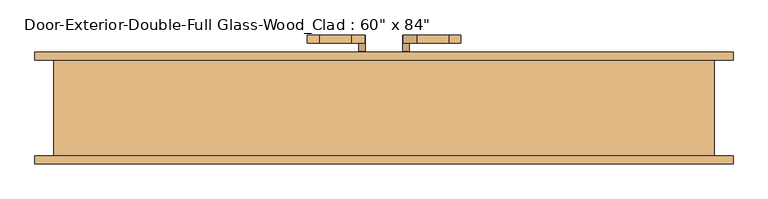
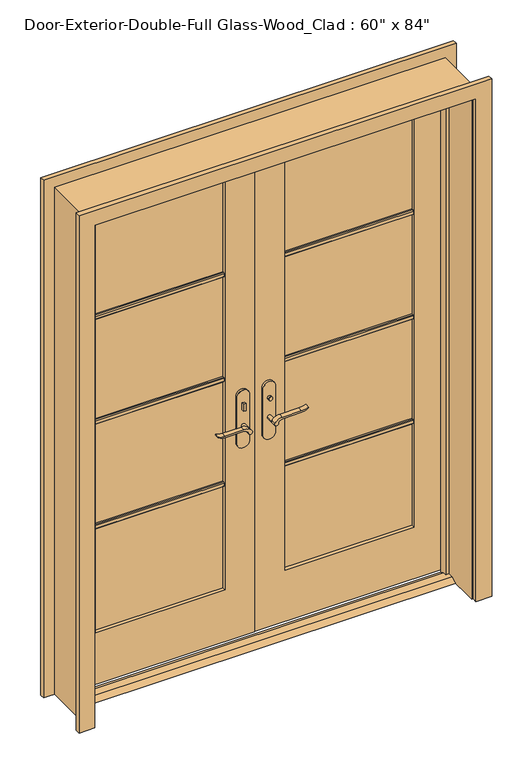
"""IFC4 building model written with IfcOpenShell, lengths in millimetres: door geometry."""

from ifc_helpers import new_model, si_unit, point, frame, frame_2d, origin, place, context, project, spatial, polyline, circle_curve, trimmed, segment, composite_curve, outline, extrude, faceted_brep, source, transform, mapped, element, save


def door_7ffae4ec(model_context):
    return source(origin(), model_context, "Body", "SolidModel", [
        extrude(outline(polyline([(19.05, 12.7), (53.975, 12.7), (79.375, 0.0), (-6.35, 0.0), (19.05, 12.7)])), frame((-762.0, 0.0, 0.0), z_axis=(1.0, 0.0, 0.0), x_axis=(0.0, 1.0, 0.0)), (0.0, 0.0, 1.0), 1524.0),
        extrude(outline(polyline([(-47.4019111, 56.2), (-57.4019111, 56.2), (-57.4019111, 66.2), (-47.4019111, 66.2), (-47.4019111, 56.2)])), frame((0.0, 0.0, 981.9), z_axis=(0.0, 0.0, 1.0), x_axis=(1.0, 0.0, 0.0)), (0.0, 0.0, 1.0), 30.0),
        extrude(outline(composite_curve([segment(trimmed(circle_curve(frame_2d((996.9, -52.4019111)), 8.0), [point((996.9, -60.4019111))], [point((996.9, -44.4019111))], False, "CARTESIAN"), True, "CONTINUOUS"), segment(trimmed(circle_curve(frame_2d((996.9, -52.4019111)), 8.0), [point((996.9, -44.4019111))], [point((996.9, -60.4019111))], False, "CARTESIAN"), True, "CONTINUOUS")], self_intersect=False)), frame((0.0, 121.125, 0.0), z_axis=(0.0, 1.0, 0.0), x_axis=(0.0, 0.0, 1.0)), (0.0, 0.0, 1.0), 10.0),
        extrude(outline(composite_curve([segment(trimmed(circle_curve(frame_2d((897.1555521, -76.0694241)), 37.2832219), [point((919.0523287, -45.8937749))], [point((934.4, -77.7693445))], False, "CARTESIAN"), True, "CONTINUOUS"), segment(polyline([(934.4, -77.7693445), (934.4, -154.045502)]), True, "CONTINUOUS"), segment(trimmed(circle_curve(frame_2d((1017.6850638, -153.9791202)), 83.2850902), [point((934.4, -154.045502))], [point((939.4, -182.4019111))], True, "CARTESIAN"), True, "CONTINUOUS"), segment(polyline([(939.4, -182.4019111), (936.6135558, -182.4019111)]), True, "CONTINUOUS"), segment(trimmed(circle_curve(frame_2d((986.6709207, -150.4622499)), 59.3791355), [point((936.6135558, -182.4019111))], [point((927.4, -154.045502))], False, "CARTESIAN"), True, "CONTINUOUS"), segment(polyline([(927.4, -154.045502), (927.4, -77.7881013)]), True, "CONTINUOUS"), segment(trimmed(circle_curve(frame_2d((909.2738613, -77.7881013)), 18.1261387), [point((927.4, -77.7881013))], [point((914.4, -60.4019111))], True, "CARTESIAN"), True, "CONTINUOUS"), segment(trimmed(circle_curve(frame_2d((914.4, -52.4019111)), 8.0), [point((914.4, -60.4019111))], [point((919.0523287, -45.8937749))], False, "CARTESIAN"), True, "CONTINUOUS")], self_intersect=False)), frame((0.0, 16.2, 0.0), z_axis=(0.0, 1.0, 0.0), x_axis=(0.0, 0.0, 1.0)), (0.0, 0.0, 1.0), 20.0),
        extrude(outline(composite_curve([segment(trimmed(circle_curve(frame_2d((914.4, -52.4019111)), 8.0), [point((914.3999903, -60.4019111))], [point((919.0523287, -45.8937749))], False, "CARTESIAN"), True, "CONTINUOUS"), segment(trimmed(circle_curve(frame_2d((897.1555521, -76.0694241)), 37.2832219), [point((919.0523287, -45.8937749))], [point((934.4, -77.7693445))], False, "CARTESIAN"), True, "CONTINUOUS"), segment(polyline([(934.4, -77.7693445), (934.4, -154.045502)]), True, "CONTINUOUS"), segment(trimmed(circle_curve(frame_2d((1017.6850638, -153.9791202)), 83.2850902), [point((934.4, -154.045502))], [point((939.4, -182.4019111))], True, "CARTESIAN"), True, "CONTINUOUS"), segment(polyline([(939.4, -182.4019111), (936.6135558, -182.4019111)]), True, "CONTINUOUS"), segment(trimmed(circle_curve(frame_2d((986.6709207, -150.4622499)), 59.3791355), [point((936.6135558, -182.4019111))], [point((927.4, -154.045502))], False, "CARTESIAN"), True, "CONTINUOUS"), segment(polyline([(927.4, -154.045502), (927.4, -77.788099)]), True, "CONTINUOUS"), segment(trimmed(circle_curve(frame_2d((909.2738682, -77.788099)), 18.1261318), [point((927.4, -77.788099))], [point((914.3999903, -60.4019111))], True, "CARTESIAN"), True, "CONTINUOUS")], self_intersect=False)), frame((0.0, 151.125, 0.0), z_axis=(0.0, 1.0, 0.0), x_axis=(0.0, 0.0, 1.0)), (0.0, 0.0, 1.0), 20.0),
        extrude(outline(composite_curve([segment(trimmed(circle_curve(frame_2d((914.4, -52.4019111)), 8.0), [point((914.4, -60.4019111))], [point((914.4, -44.4019111))], False, "CARTESIAN"), True, "CONTINUOUS"), segment(trimmed(circle_curve(frame_2d((914.4, -52.4019111)), 8.0), [point((914.4, -44.4019111))], [point((914.4, -60.4019111))], False, "CARTESIAN"), True, "CONTINUOUS")], self_intersect=False)), frame((0.0, 36.2, 0.0), z_axis=(0.0, 1.0, 0.0), x_axis=(0.0, 0.0, 1.0)), (0.0, 0.0, 1.0), 30.0),
        extrude(outline(composite_curve([segment(trimmed(circle_curve(frame_2d((914.4, -52.4019111)), 8.0), [point((914.4, -60.4019111))], [point((914.4, -44.4019111))], False, "CARTESIAN"), True, "CONTINUOUS"), segment(trimmed(circle_curve(frame_2d((914.4, -52.4019111)), 8.0), [point((914.4, -44.4019111))], [point((914.4, -60.4019111))], False, "CARTESIAN"), True, "CONTINUOUS")], self_intersect=False)), frame((0.0, 121.125, 0.0), z_axis=(0.0, 1.0, 0.0), x_axis=(0.0, 0.0, 1.0)), (0.0, 0.0, 1.0), 30.0),
        extrude(outline(composite_curve([segment(polyline([(844.4, -27.4019111), (1039.4, -27.4019111)]), True, "CONTINUOUS"), segment(trimmed(circle_curve(frame_2d((1039.4, -52.4019111)), 25.0), [point((1039.4, -27.4019111))], [point((1039.4, -77.4019111))], False, "CARTESIAN"), True, "CONTINUOUS"), segment(polyline([(1039.4, -77.4019111), (844.4, -77.4019111)]), True, "CONTINUOUS"), segment(trimmed(circle_curve(frame_2d((844.4, -52.4019111)), 25.0), [point((844.4, -77.4019111))], [point((844.4, -27.4019111))], False, "CARTESIAN"), True, "CONTINUOUS")], self_intersect=False)), frame((0.0, 66.2, 0.0), z_axis=(0.0, 1.0, 0.0), x_axis=(0.0, 0.0, 1.0)), (0.0, 0.0, 1.0), 10.0),
        extrude(outline(composite_curve([segment(polyline([(844.4, -27.4019111), (1039.4, -27.4019111)]), True, "CONTINUOUS"), segment(trimmed(circle_curve(frame_2d((1039.4, -52.4019111)), 25.0), [point((1039.4, -27.4019111))], [point((1039.4, -77.4019111))], False, "CARTESIAN"), True, "CONTINUOUS"), segment(polyline([(1039.4, -77.4019111), (844.4, -77.4019111)]), True, "CONTINUOUS"), segment(trimmed(circle_curve(frame_2d((844.4, -52.4019111)), 25.0), [point((844.4, -77.4019111))], [point((844.4, -27.4019111))], False, "CARTESIAN"), True, "CONTINUOUS")], self_intersect=False)), frame((0.0, 111.125, 0.0), z_axis=(0.0, 1.0, 0.0), x_axis=(0.0, 0.0, 1.0)), (0.0, 0.0, 1.0), 10.0),
        extrude(outline(polyline([(47.3875, 131.125), (57.3875, 131.125), (57.3875, 121.125), (47.3875, 121.125), (47.3875, 131.125)])), frame((0.0, 0.0, 981.9), z_axis=(0.0, 0.0, 1.0), x_axis=(1.0, 0.0, 0.0)), (0.0, 0.0, 1.0), 30.0),
        extrude(outline(composite_curve([segment(trimmed(circle_curve(frame_2d((996.9, 52.3875)), 8.0), [point((996.9, 60.3875))], [point((996.9, 44.3875))], False, "CARTESIAN"), True, "CONTINUOUS"), segment(trimmed(circle_curve(frame_2d((996.9, 52.3875)), 8.0), [point((996.9, 44.3875))], [point((996.9, 60.3875))], False, "CARTESIAN"), True, "CONTINUOUS")], self_intersect=False)), frame((0.0, 56.2, 0.0), z_axis=(0.0, 1.0, 0.0), x_axis=(0.0, 0.0, 1.0)), (0.0, 0.0, 1.0), 10.0),
        extrude(outline(composite_curve([segment(trimmed(circle_curve(frame_2d((914.4, 52.3875)), 8.0), [point((919.0523287, 45.8793637))], [point((914.4, 60.3875))], False, "CARTESIAN"), True, "CONTINUOUS"), segment(trimmed(circle_curve(frame_2d((909.2738613, 77.7736901)), 18.1261387), [point((914.4, 60.3875))], [point((927.4, 77.7736901))], True, "CARTESIAN"), True, "CONTINUOUS"), segment(polyline([(927.4, 77.7736901), (927.4, 154.0310909)]), True, "CONTINUOUS"), segment(trimmed(circle_curve(frame_2d((986.6709207, 150.4478388)), 59.3791355), [point((927.4, 154.0310909))], [point((936.6135558, 182.3875))], False, "CARTESIAN"), True, "CONTINUOUS"), segment(polyline([(936.6135558, 182.3875), (939.4, 182.3875)]), True, "CONTINUOUS"), segment(trimmed(circle_curve(frame_2d((1017.6850638, 153.9647091)), 83.2850902), [point((939.4, 182.3875))], [point((934.4, 154.0310909))], True, "CARTESIAN"), True, "CONTINUOUS"), segment(polyline([(934.4, 154.0310909), (934.4, 77.7549333)]), True, "CONTINUOUS"), segment(trimmed(circle_curve(frame_2d((897.1555521, 76.0550129)), 37.2832219), [point((934.4, 77.7549333))], [point((919.0523287, 45.8793637))], False, "CARTESIAN"), True, "CONTINUOUS")], self_intersect=False)), frame((0.0, 151.125, 0.0), z_axis=(0.0, 1.0, 0.0), x_axis=(0.0, 0.0, 1.0)), (0.0, 0.0, 1.0), 20.0),
        extrude(outline(composite_curve([segment(trimmed(circle_curve(frame_2d((909.2738682, 77.7736878)), 18.1261318), [point((914.3999903, 60.3875))], [point((927.4, 77.7736878))], True, "CARTESIAN"), True, "CONTINUOUS"), segment(polyline([(927.4, 77.7736878), (927.4, 154.0310909)]), True, "CONTINUOUS"), segment(trimmed(circle_curve(frame_2d((986.6709207, 150.4478388)), 59.3791355), [point((927.4, 154.0310909))], [point((936.6135558, 182.3875))], False, "CARTESIAN"), True, "CONTINUOUS"), segment(polyline([(936.6135558, 182.3875), (939.4, 182.3875)]), True, "CONTINUOUS"), segment(trimmed(circle_curve(frame_2d((1017.6850638, 153.9647091)), 83.2850902), [point((939.4, 182.3875))], [point((934.4, 154.0310909))], True, "CARTESIAN"), True, "CONTINUOUS"), segment(polyline([(934.4, 154.0310909), (934.4, 77.7549333)]), True, "CONTINUOUS"), segment(trimmed(circle_curve(frame_2d((897.1555521, 76.0550129)), 37.2832219), [point((934.4, 77.7549333))], [point((919.0523287, 45.8793637))], False, "CARTESIAN"), True, "CONTINUOUS"), segment(trimmed(circle_curve(frame_2d((914.4, 52.3875)), 8.0), [point((919.0523287, 45.8793637))], [point((914.3999903, 60.3875))], False, "CARTESIAN"), True, "CONTINUOUS")], self_intersect=False)), frame((0.0, 16.2, 0.0), z_axis=(0.0, 1.0, 0.0), x_axis=(0.0, 0.0, 1.0)), (0.0, 0.0, 1.0), 20.0),
        extrude(outline(composite_curve([segment(trimmed(circle_curve(frame_2d((914.4, 52.3875)), 8.0), [point((914.4, 60.3875))], [point((914.4, 44.3875))], False, "CARTESIAN"), True, "CONTINUOUS"), segment(trimmed(circle_curve(frame_2d((914.4, 52.3875)), 8.0), [point((914.4, 44.3875))], [point((914.4, 60.3875))], False, "CARTESIAN"), True, "CONTINUOUS")], self_intersect=False)), frame((0.0, 121.125, 0.0), z_axis=(0.0, 1.0, 0.0), x_axis=(0.0, 0.0, 1.0)), (0.0, 0.0, 1.0), 30.0),
        extrude(outline(composite_curve([segment(trimmed(circle_curve(frame_2d((914.4, 52.3875)), 8.0), [point((914.4, 60.3875))], [point((914.4, 44.3875))], False, "CARTESIAN"), True, "CONTINUOUS"), segment(trimmed(circle_curve(frame_2d((914.4, 52.3875)), 8.0), [point((914.4, 44.3875))], [point((914.4, 60.3875))], False, "CARTESIAN"), True, "CONTINUOUS")], self_intersect=False)), frame((0.0, 36.2, 0.0), z_axis=(0.0, 1.0, 0.0), x_axis=(0.0, 0.0, 1.0)), (0.0, 0.0, 1.0), 30.0),
        extrude(outline(composite_curve([segment(trimmed(circle_curve(frame_2d((844.4, 52.3875)), 25.0), [point((844.4, 27.3875))], [point((844.4, 77.3875))], False, "CARTESIAN"), True, "CONTINUOUS"), segment(polyline([(844.4, 77.3875), (1039.4, 77.3875)]), True, "CONTINUOUS"), segment(trimmed(circle_curve(frame_2d((1039.4, 52.3875)), 25.0), [point((1039.4, 77.3875))], [point((1039.4, 27.3875))], False, "CARTESIAN"), True, "CONTINUOUS"), segment(polyline([(1039.4, 27.3875), (844.4, 27.3875)]), True, "CONTINUOUS")], self_intersect=False)), frame((0.0, 111.125, 0.0), z_axis=(0.0, 1.0, 0.0), x_axis=(0.0, 0.0, 1.0)), (0.0, 0.0, 1.0), 10.0),
        extrude(outline(composite_curve([segment(trimmed(circle_curve(frame_2d((844.4, 52.3875)), 25.0), [point((844.4, 27.3875))], [point((844.4, 77.3875))], False, "CARTESIAN"), True, "CONTINUOUS"), segment(polyline([(844.4, 77.3875), (1039.4, 77.3875)]), True, "CONTINUOUS"), segment(trimmed(circle_curve(frame_2d((1039.4, 52.3875)), 25.0), [point((1039.4, 77.3875))], [point((1039.4, 27.3875))], False, "CARTESIAN"), True, "CONTINUOUS"), segment(polyline([(1039.4, 27.3875), (844.4, 27.3875)]), True, "CONTINUOUS")], self_intersect=False)), frame((0.0, 66.2, 0.0), z_axis=(0.0, 1.0, 0.0), x_axis=(0.0, 0.0, 1.0)), (0.0, 0.0, 1.0), 10.0),
        extrude(outline(polyline([(90.17, 1578.371875), (90.17, 1559.321875), (83.82, 1559.321875), (80.645, 1562.496875), (80.645, 1575.196875), (83.82, 1578.371875), (90.17, 1578.371875)])), frame((120.65, 0.0, 0.0), z_axis=(1.0, 0.0, 0.0), x_axis=(0.0, 1.0, 0.0)), (0.0, 0.0, 1.0), 520.7),
        extrude(outline(polyline([(90.17, 1132.68125), (90.17, 1113.63125), (83.82, 1113.63125), (80.645, 1116.80625), (80.645, 1129.50625), (83.82, 1132.68125), (90.17, 1132.68125)])), frame((120.65, 0.0, 0.0), z_axis=(1.0, 0.0, 0.0), x_axis=(0.0, 1.0, 0.0)), (0.0, 0.0, 1.0), 520.7),
        extrude(outline(polyline([(90.17, 686.990625), (90.17, 667.940625), (83.82, 667.940625), (80.645, 671.115625), (80.645, 683.815625), (83.82, 686.990625), (90.17, 686.990625)])), frame((120.65, 0.0, 0.0), z_axis=(1.0, 0.0, 0.0), x_axis=(0.0, 1.0, 0.0)), (0.0, 0.0, 1.0), 520.7),
        extrude(outline(polyline([(97.155, 1578.371875), (103.505, 1578.371875), (106.68, 1575.196875), (106.68, 1562.496875), (103.505, 1559.321875), (97.155, 1559.321875), (97.155, 1578.371875)])), frame((-641.35, 0.0, 0.0), z_axis=(1.0, 0.0, 0.0), x_axis=(0.0, 1.0, 0.0)), (0.0, 0.0, 1.0), 520.7),
        extrude(outline(polyline([(97.155, 1132.68125), (103.505, 1132.68125), (106.68, 1129.50625), (106.68, 1116.80625), (103.505, 1113.63125), (97.155, 1113.63125), (97.155, 1132.68125)])), frame((-641.35, 0.0, 0.0), z_axis=(1.0, 0.0, 0.0), x_axis=(0.0, 1.0, 0.0)), (0.0, 0.0, 1.0), 520.7),
        extrude(outline(polyline([(97.155, 686.990625), (103.505, 686.990625), (106.68, 683.815625), (106.68, 671.115625), (103.505, 667.940625), (97.155, 667.940625), (97.155, 686.990625)])), frame((-641.35, 0.0, 0.0), z_axis=(1.0, 0.0, 0.0), x_axis=(0.0, 1.0, 0.0)), (0.0, 0.0, 1.0), 520.7),
        extrude(outline(polyline([(97.155, 1578.371875), (103.505, 1578.371875), (106.68, 1575.196875), (106.68, 1562.496875), (103.505, 1559.321875), (97.155, 1559.321875), (97.155, 1578.371875)])), frame((120.65, 0.0, 0.0), z_axis=(1.0, 0.0, 0.0), x_axis=(0.0, 1.0, 0.0)), (0.0, 0.0, 1.0), 520.7),
        extrude(outline(polyline([(97.155, 1132.68125), (103.505, 1132.68125), (106.68, 1129.50625), (106.68, 1116.80625), (103.505, 1113.63125), (97.155, 1113.63125), (97.155, 1132.68125)])), frame((120.65, 0.0, 0.0), z_axis=(1.0, 0.0, 0.0), x_axis=(0.0, 1.0, 0.0)), (0.0, 0.0, 1.0), 520.7),
        extrude(outline(polyline([(97.155, 686.990625), (103.505, 686.990625), (106.68, 683.815625), (106.68, 671.115625), (103.505, 667.940625), (97.155, 667.940625), (97.155, 686.990625)])), frame((120.65, 0.0, 0.0), z_axis=(1.0, 0.0, 0.0), x_axis=(0.0, 1.0, 0.0)), (0.0, 0.0, 1.0), 520.7),
        extrude(outline(polyline([(90.17, 1578.371875), (90.17, 1559.321875), (83.82, 1559.321875), (80.645, 1562.496875), (80.645, 1575.196875), (83.82, 1578.371875), (90.17, 1578.371875)])), frame((-641.35, 0.0, 0.0), z_axis=(1.0, 0.0, 0.0), x_axis=(0.0, 1.0, 0.0)), (0.0, 0.0, 1.0), 520.7),
        extrude(outline(polyline([(90.17, 1132.68125), (90.17, 1113.63125), (83.82, 1113.63125), (80.645, 1116.80625), (80.645, 1129.50625), (83.82, 1132.68125), (90.17, 1132.68125)])), frame((-641.35, 0.0, 0.0), z_axis=(1.0, 0.0, 0.0), x_axis=(0.0, 1.0, 0.0)), (0.0, 0.0, 1.0), 520.7),
        extrude(outline(polyline([(90.17, 686.990625), (90.17, 667.940625), (83.82, 667.940625), (80.645, 671.115625), (80.645, 683.815625), (83.82, 686.990625), (90.17, 686.990625)])), frame((-641.35, 0.0, 0.0), z_axis=(1.0, 0.0, 0.0), x_axis=(0.0, 1.0, 0.0)), (0.0, 0.0, 1.0), 520.7),
        extrude(outline(polyline([(0.0, 768.35), (0.0, 831.85), (2203.45, 831.85), (2203.45, -831.85), (0.0, -831.85), (0.0, -768.35), (2139.95, -768.35), (2139.95, 768.35), (0.0, 768.35)])), frame((0.0, -136.525, 0.0), z_axis=(0.0, 1.0, 0.0), x_axis=(0.0, 0.0, 1.0)), (0.0, 0.0, 1.0), 19.05),
        extrude(outline(polyline([(0.0, 768.35), (0.0, 831.85), (2203.45, 831.85), (2203.45, -831.85), (0.0, -831.85), (0.0, -768.35), (2139.95, -768.35), (2139.95, 768.35), (0.0, 768.35)])), frame((0.0, 111.125, 0.0), z_axis=(0.0, 1.0, 0.0), x_axis=(0.0, 0.0, 1.0)), (0.0, 0.0, 1.0), 19.05),
        faceted_brep([(787.4, 111.125, 0.0), (787.4, -117.475, 0.0), (762.0, -117.475, 0.0), (762.0, 41.275, 0.0), (749.3, 41.275, 0.0), (749.3, 76.2, 0.0), (762.0, 76.2, 0.0), (762.0, 111.125, 0.0), (787.4, 111.125, 2159.0), (787.4, -117.475, 2159.0), (-787.4, -117.475, 2159.0), (-787.4, -117.475, 0.0), (-762.0, -117.475, 0.0), (-762.0, -117.475, 2133.6), (762.0, -117.475, 2133.6), (762.0, 41.275, 2133.6), (-762.0, 41.275, 2133.6), (-762.0, 41.275, 0.0), (-749.3, 41.275, 0.0), (-749.3, 41.275, 2120.9), (749.3, 41.275, 2120.9), (749.3, 76.2, 2120.9), (1.5875, 76.2, 2120.9), (-1.6019111, 76.2, 2120.9), (-749.3, 76.2, 2120.9), (-749.3, 76.2, 0.0), (-762.0, 76.2, 0.0), (-762.0, 76.2, 2133.6), (-1.6019111, 76.2, 2133.6), (1.5875, 76.2, 2133.6), (762.0, 76.2, 2133.6), (762.0, 111.125, 2133.6), (1.5875, 111.125, 2133.6), (-1.6019111, 111.125, 2133.6), (-762.0, 111.125, 2133.6), (-762.0, 111.125, 0.0), (-787.4, 111.125, 0.0), (-787.4, 111.125, 2159.0)], [[[0, 1, 2, 3, 4, 5, 6, 7]], [[1, 0, 8, 9]], [[2, 1, 9, 10, 11, 12, 13, 14]], [[3, 2, 14, 15]], [[4, 3, 15, 16, 17, 18, 19, 20]], [[5, 4, 20, 21]], [[6, 5, 21, 22, 23, 24, 25, 26, 27, 28, 29, 30]], [[7, 6, 30, 31]], [[0, 7, 31, 32, 33, 34, 35, 36, 37, 8]], [[9, 8, 37, 10]], [[14, 13, 16, 15]], [[20, 19, 24, 23, 22, 21]], [[31, 30, 29, 28, 27, 34, 33, 32]], [[12, 11, 36, 35, 26, 25, 18, 17]], [[11, 10, 37, 36]], [[13, 12, 17, 16]], [[19, 18, 25, 24]], [[27, 26, 35, 34]]]),
        extrude(outline(polyline([(12.7, 762.0), (2133.6, 762.0), (2133.6, 1.5875), (12.7, 1.5875), (12.7, 762.0)]), holes=[polyline([(2014.5375, 120.65), (2014.5375, 641.35), (231.775, 641.35), (231.775, 120.65), (2014.5375, 120.65)])]), frame((0.0, 76.2, 0.0), z_axis=(0.0, 1.0, 0.0), x_axis=(0.0, 0.0, 1.0)), (0.0, 0.0, 1.0), 34.925),
        extrude(outline(polyline([(2133.6, -762.0), (12.7, -762.0), (12.7, -1.6019111), (2133.6, -1.6019111), (2133.6, -762.0)]), holes=[polyline([(231.775, -641.35), (2014.5375, -641.35), (2014.5375, -120.65), (231.775, -120.65), (231.775, -641.35)])]), frame((0.0, 76.2, 0.0), z_axis=(0.0, 1.0, 0.0), x_axis=(0.0, 0.0, 1.0)), (0.0, 0.0, 1.0), 34.925),
        extrude(outline(polyline([(641.35, 90.17), (120.65, 90.17), (120.65, 97.155), (641.35, 97.155), (641.35, 90.17)])), frame((0.0, 0.0, 231.775), z_axis=(0.0, 0.0, 1.0), x_axis=(1.0, 0.0, 0.0)), (0.0, 0.0, 1.0), 1782.7625),
        extrude(outline(polyline([(-120.65, 90.17), (-641.35, 90.17), (-641.35, 97.155), (-120.65, 97.155), (-120.65, 90.17)])), frame((0.0, 0.0, 231.775), z_axis=(0.0, 0.0, 1.0), x_axis=(1.0, 0.0, 0.0)), (0.0, 0.0, 1.0), 1782.7625),
    ])


if __name__ == "__main__":
    model = new_model("IFC4")
    model_context = context("Model", 3, world=origin())
    ifc_project = project(units=[si_unit("LENGTHUNIT", "METRE", prefix="MILLI")], contexts=[model_context])
    site = spatial("IfcSite", under=ifc_project)
    building = spatial("IfcBuilding", under=site)
    placement = place(None, origin())
    door_shape = door_7ffae4ec(model_context)
    element("IfcDoor", 1, ObjectType="Door-Exterior-Double-Full Glass-Wood_Clad : 60\" x 84\"", at=placement, inside=building, context=model_context, shape_type="MappedRepresentation", body=[
        mapped(door_shape, transform((0.0, 0.0, 0.0), x_axis=(1.0, 0.0, 0.0), y_axis=(0.0, 1.0, 0.0), z_axis=(0.0, 0.0, 1.0))),
    ])
    save(model, "model.ifc")

# Revit data of these elements
# Type "Door-Exterior-Double-Full Glass-Wood_Clad : 60\" x 84\""
#   Type Mark = "8"
#   Assembly Code = "B2030100"
#   Analytic Construction = "French door, wood frame with double glass"
#   Top Rail = 0' - 4 11/16"
#   Threshold Offset [instance default] = 0' - 0 1/2"
#   Thickness = 0' - 1 3/8"
#   Thermal Resistance (R) = 1.9158 (h·ft²·°F)/BTU
#   Swing Angle [instance default] = 90.00°
#   Stiles = 0' - 4 3/4"
#   Rough Width = 5' - 2"
#   Rough Height = 7' - 1"
#   Panel Width = 2' - 6"
#   Door Offset [instance default] = 0' - 0"
#   Height = 7' - 0"
#   Width = 5' - 0"
#   Heat Transfer Coefficient (U) = 0.5220 BTU/(h·ft²·°F)
#   Bottom Rail = 0' - 9 1/8"
#   Exterior Trim [instance default] = yes
#   Threshold [instance default] = yes
#   Show Grill [instance default] = yes
#   Function = 1
#   Trim Material = Cherry
#   Threshold Material = Cherry
#   Panel Material = Cherry
#   Glazing = Glass
#   Frame Material = Cherry
#   Door Handle Material = Aluminum
#   Visual Light Transmittance = 0
#   Solar Heat Gain Coefficient = 0
#   Wall Closure = (empty or 0)
#   Construction Type = (empty or 0)
# Element 1 (IfcDoor, "Door-Exterior-Double-Full Glass-Wood_Clad : 60\" x 84\"")
#   Materials on its faces: "Cherry", "Aluminum", "Glass"
# Materials
#   "Cherry": class "Wood", colour RGB 226 177 128, transparency 0, Description = "Prunus Serotina", Cost = 0
#   "Glass": class "Glass", colour RGB 0 128 192, transparency 0.75, Description = "Soda Lime Glass", Cost = 0
#   "Aluminum": class "Metal", colour RGB 247 247 247, transparency 0, Description = "Aluminum 6061", Cost = 0
